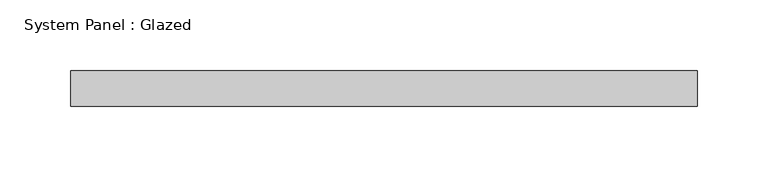
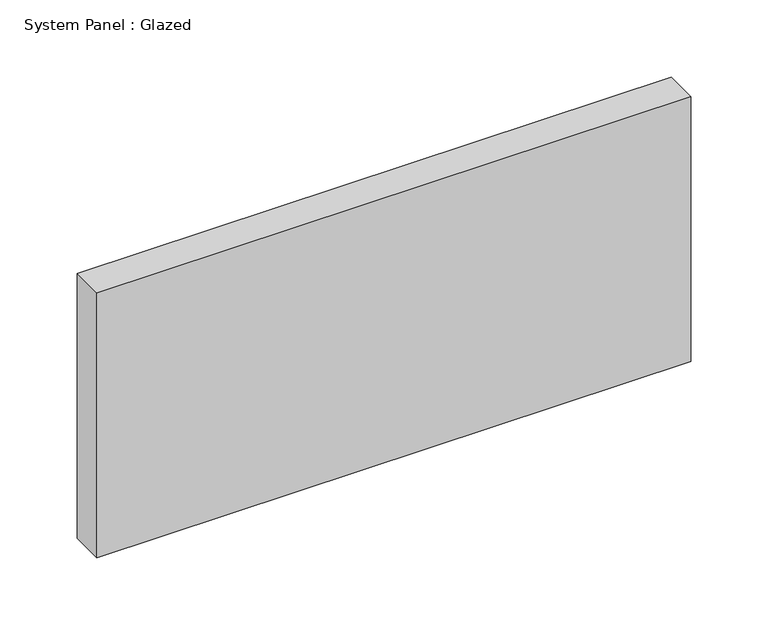
"""IFC4 building model written with IfcOpenShell, lengths in millimetres: plate geometry, System Panel : Glazed."""

from ifc_helpers import new_model, si_unit, origin, origin_with_axes, place, context, project, spatial, polyline, outline, extrude, source, transform, mapped, element, save


def system_panel_glazed_c196d27b(model_context):
    return source(origin(), model_context, "Body", "SweptSolid", [
        extrude(outline(polyline([(222.25, 19.05), (-222.25, 19.05), (-222.25, 44.45), (222.25, 44.45), (222.25, 19.05)])), origin_with_axes(), (0.0, 0.0, 1.0), 209.55),
    ])


if __name__ == "__main__":
    model = new_model("IFC4")
    model_context = context("Model", 3, world=origin())
    ifc_project = project(units=[si_unit("LENGTHUNIT", "METRE", prefix="MILLI")], contexts=[model_context])
    site = spatial("IfcSite", under=ifc_project)
    building = spatial("IfcBuilding", under=site)
    placement = place(None, origin())
    system_panel_glazed_shape = system_panel_glazed_c196d27b(model_context)
    element("IfcPlate", 1, ObjectType="System Panel : Glazed", at=placement, inside=building, context=model_context, shape_type="MappedRepresentation", body=[
        mapped(system_panel_glazed_shape, transform((0.0, 0.0, 0.0), x_axis=(1.0, 0.0, 0.0), y_axis=(0.0, 1.0, 0.0), z_axis=(0.0, 0.0, 1.0))),
    ])
    save(model, "model.ifc")

# Revit data of these elements
# Type "System Panel : Glazed"
#   Construction Type Id = "GSP4R"
#   Analytic Construction = "1/8 in Pilkington single glazing"
#   Visual Light Transmittance = 0.9
#   Solar Heat Gain Coefficient = 0.86
#   Heat Transfer Coefficient (U) = 1.18115 BTU/(h·ft²·°F)
#   Define Thermal Properties by = 1
# Element 1 (IfcPlate, "System Panel : Glazed")
#   Materials on its faces: "Glass"
# Materials
#   "Glass": class "Glass", colour RGB 0 128 192, transparency 0.75, Description = "Soda Lime Glass", Cost = 0
